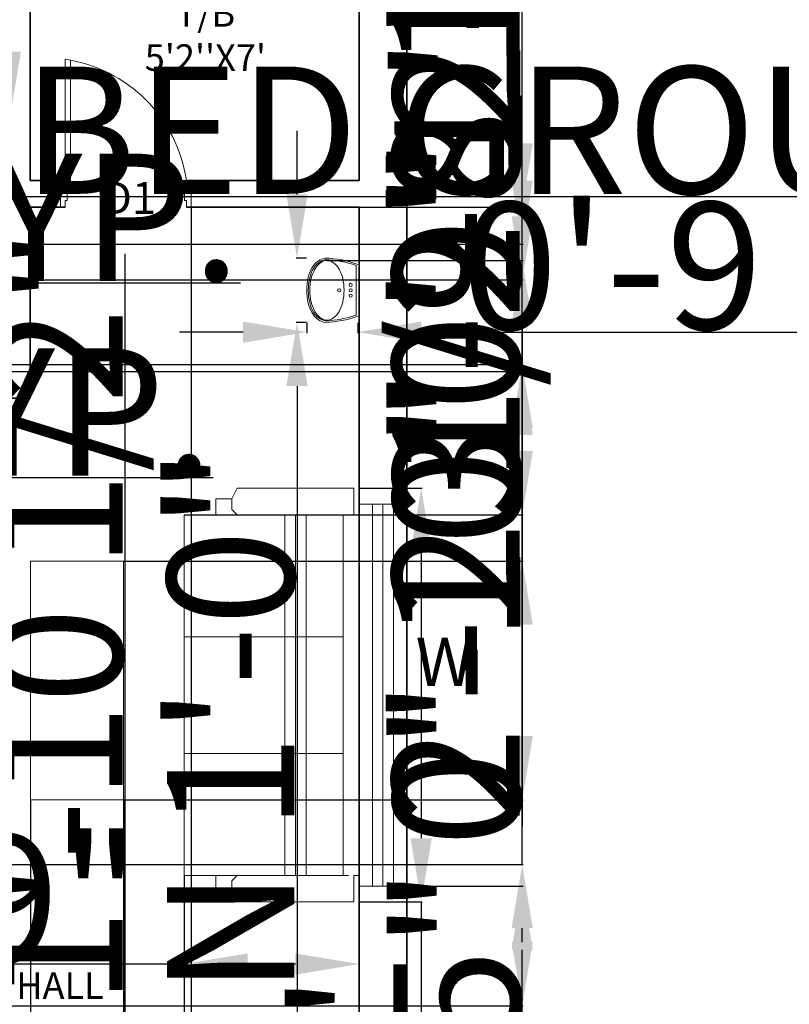
# Model space of a CAD drawing. Units: inches. Extents: x 2236 to 2927, y 1577 to 2452.
# Tile 6 of 9: x 2550 to 2695, y 1836 to 2021. Entities that reach past the tile are written whole.
import ezdxf

# ---------------------------------------------------------------- set-up
doc = ezdxf.new("R2010")
doc.units = ezdxf.units.IN
for name, color, linetype, lineweight in [('A-ANNO-DIMS', 2, 'Continuous', 18), ('A-ANNO-TEXT', 7, 'Continuous', 18), ('A-AREA-IDEN', 7, 'Continuous', 18), ('A-FLOR-FIXT', 9, 'Continuous', 18), ('A-FURN', 8, 'Continuous', 18), ('Doors', 150, 'Continuous', 18), ('Wall', 7, 'Continuous', 35), ('Windows', 162, 'Continuous', 18)]:
    doc.layers.add(name, color=color, linetype=linetype, lineweight=lineweight)
doc.styles.get("Standard").update_dxf_attribs({"font": 'arial.ttf'})
doc.dimstyles.get("Standard").update_dxf_attribs({"dimtxt": 24, "dimasz": 12, "dimexe": 0.18, "dimexo": 0.0625, "dimgap": 0.09, "dimtad": 1, "dimdec": 1, "dimzin": 0, "dimdsep": 46, "dimlunit": 4, "dimtxsty": 'Standard', "dimcen": 0.09, "dimadec": 0, "dimazin": 0, "dimtfac": 1, "dimtdec": 1, "dimtofl": 0, "dimtmove": 0, "dimatfit": 3, "dimfxl": 1, "dimtolj": 1, "dimtzin": 0, "dimarcsym": 0})

# ---------------------------------------------------------------- blocks, each defined once
blk = doc.blocks.new('wash-3')
at = {"color": 0, "linetype": 'ByBlock'}
blk.add_line((0.2303, -0.0146), (-0.2303, -0.0146), dxfattribs=at)
for centre in [(-0.05, -0.0656), (0, -0.0656), (0.05, -0.0656), (0, -0.1721)]:
    blk.add_circle(centre, 0.0148, dxfattribs=at)
for centre, radius, start, end in [((0.6901, -0.3398), 0.9908, 159.94105, 177.83899), ((0.6901, -0.3398), 0.9762, 160.53992, 177.73258), ((-0.6901, -0.3398), 0.9762, 2.26742, 19.46008), ((-0.6901, -0.3398), 0.9908, 2.16101, 20.05895), ((-0.0958, -0.3493), 0.2026, 119.83217, 144.15878), ((-0.038, -0.4501), 0.3188, 103.36192, 119.83217), ((0, -0.6101), 0.4833, 90, 103.36192), ((0, -0.6101), 0.4833, 76.63808, 90), ((0.038, -0.4501), 0.3188, 60.16783, 76.63808), ((0.0958, -0.3493), 0.2026, 35.84122, 60.16783), ((-0.1831, -0.2863), 0.095, 144.15878, 180), ((0.1831, -0.2863), 0.095, 0, 35.84122), ((-0.12, -0.2651), 0.1838, 191.74238, 233.41914), ((-0.12, -0.2651), 0.1692, 192.33583, 233.36097), ((-0.1831, -0.2863), 0.095, 180, 215.84122), ((-0.0958, -0.2233), 0.2026, 215.84122, 240.16783), ((0.0958, -0.2233), 0.2026, 299.83217, 324.15878), ((0.12, -0.2651), 0.1692, 306.63903, 347.66417), ((0.12, -0.2651), 0.1838, 306.58086, 348.25762), ((0.1831, -0.2863), 0.095, 324.15878, 0), ((-0.0958, -0.2233), 0.2319, 234.77185, 240.16783), ((-0.0958, -0.2233), 0.2173, 234.81756, 240.16783), ((-0.038, -0.1224), 0.3481, 240.16783, 256.63808), ((-0.038, -0.1224), 0.3335, 240.16783, 256.63808), ((-0.038, -0.1224), 0.3188, 240.16783, 256.63808), ((0, 0.0376), 0.4979, 256.63808, 270), ((0, 0.0376), 0.4833, 256.63808, 270), ((0, 0.0376), 0.4833, 270, 283.36192), ((0, 0.0376), 0.4979, 270, 283.36192), ((0.038, -0.1224), 0.3188, 283.36192, 299.83217), ((0.038, -0.1224), 0.3335, 283.36192, 299.83217), ((0.038, -0.1224), 0.3481, 283.36192, 299.83217), ((0.0958, -0.2233), 0.2173, 299.83217, 305.18244), ((0.0958, -0.2233), 0.2319, 299.83217, 305.22815), ((0, 0.0376), 0.5126, 256.63808, 270), ((0, 0.0376), 0.5126, 270, 283.36192)]:
    blk.add_arc(centre, radius, start, end, dxfattribs=at)
blk = doc.blocks.new('12PCOU13')
at = {"color": 0, "linetype": 'ByBlock'}
for p, q in [((24, 37), (24, 35)), ((23, 34), (2, 34)), ((3, -34), (3, 34)), ((10, 34), (10, -34)), ((12, 34), (12, -34)), ((14, 34), (14, -34)), ((24, 35), (23, 34)), ((27, 34), (23, 34)), ((33, 11), (3, 11)), ((33, -11), (3, -11)), ((23, -34), (2, -34)), ((27, -34), (23, -34)), ((24, -35), (23, -34)), ((24, -37), (24, -35))]:
    blk.add_line(p, q, dxfattribs=at)
blk.add_lwpolyline([(1, -39), (1, -34), (0, -34), (0, 34), (1, 34), (1, 39), (23, 39), (24, 37), (27, 37), (27, 34), (33, 34), (33, -34), (27, -34), (27, -37), (24, -37), (23, -39)], close=True, dxfattribs=at)
blk = doc.blocks.new('AP0B07')
for p, q in [((33.6, 96), (33.6, 978.8)), ((72, 96), (72, 972.3)), ((0, 96), (0, -96)), ((33.6, 96), (0, 96)), ((33.6, 48), (33.6, 96)), ((48, 48), (33.6, 48)), ((48, -48), (48, 48)), ((33.6, -96), (33.6, -48)), ((33.6, -48), (48, -48)), ((0, -96), (33.6, -96))]:
    blk.add_line(p, q)
blk.add_lwpolyline([(33.6, 96), (72, 96)])
blk.add_lwpolyline([(950, 96), (950, -96), (916.4, -96), (916.4, -48), (902, -48), (902, 48), (916.4, 48), (916.4, 96)], close=True)
blk.add_arc((-123.6, -61.2), 1051.8, 8.59637, 81.40363)
blk = doc.blocks.new('WIN-72IN')
for p, q in [((0, 6.5), (72, 6.5)), ((0, 4.5), (72, 4.5)), ((0, 2.5), (72, 2.5))]:
    blk.add_line(p, q)
blk.add_lwpolyline([(0, 9), (72, 9), (72, 0), (0, 0)], close=True)
blk = doc.blocks.new('*D17')
at = {"layer": 'A-ANNO-DIMS', "color": 0, "lineweight": -2, "transparency": 16777216}
for p, q in [((2405.85, 1971.79), (2393.85, 1971.79)), ((2417.85, 1972.28), (2417.85, 1971.61)), ((2420.99, 1972.28), (2420.99, 1971.61)), ((2432.99, 1971.79), (2591.46, 1971.79))]:
    blk.add_line(p, q, dxfattribs=at)
at = {"layer": 'A-ANNO-DIMS', "color": 0, "transparency": 16777216}
for points in [[(2405.85, 1973.79), (2405.85, 1969.79), (2417.85, 1971.79)], [(2432.99, 1973.79), (2432.99, 1969.79), (2420.99, 1971.79)]]:
    blk.add_solid(points, dxfattribs=at)
at = {"layer": 'Defpoints', "color": 0, "transparency": 16777216}
for p in [(2417.85, 1972.34), (2420.99, 1972.34), (2420.99, 1971.79)]:
    blk.add_point(p, dxfattribs=at)
at = {"layer": 'A-ANNO-DIMS', "color": 0, "transparency": 16777216, "insert": (2518.23, 1984.14), "char_height": 24, "attachment_point": 5}
blk.add_mtext('\\A1;0\'-3" TYP.', dxfattribs=at)
blk = doc.blocks.new('*D21')
at = {"layer": 'A-ANNO-DIMS', "color": 0, "lineweight": -2, "transparency": 16777216}
for p, q in [((2394.85, 1935.11), (2382.85, 1935.11)), ((2406.85, 1929.77), (2406.85, 1935.29)), ((2415.85, 1929.77), (2415.85, 1935.29)), ((2427.85, 1935.11), (2586.32, 1935.11))]:
    blk.add_line(p, q, dxfattribs=at)
at = {"layer": 'A-ANNO-DIMS', "color": 0, "transparency": 16777216}
for points in [[(2394.85, 1937.11), (2394.85, 1933.11), (2406.85, 1935.11)], [(2427.85, 1937.11), (2427.85, 1933.11), (2415.85, 1935.11)]]:
    blk.add_solid(points, dxfattribs=at)
at = {"layer": 'Defpoints', "color": 0, "transparency": 16777216}
for p in [(2415.85, 1935.11), (2406.85, 1929.71), (2415.85, 1929.71)]:
    blk.add_point(p, dxfattribs=at)
at = {"layer": 'A-ANNO-DIMS', "color": 0, "transparency": 16777216, "insert": (2513.08, 1947.45), "char_height": 24, "attachment_point": 5}
blk.add_mtext('\\A1;0\'-9" TYP.', dxfattribs=at)
blk = doc.blocks.new('*D22')
at = {"layer": 'A-ANNO-DIMS', "color": 0, "lineweight": -2, "transparency": 16777216}
for p, q in [((2514.42, 1977.96), (2514.42, 2358.7)), ((2518.53, 1977.96), (2514.24, 1977.96)), ((2514.42, 1962.08), (2514.42, 1965.96)), ((2518.53, 1950.08), (2514.24, 1950.08))]:
    blk.add_line(p, q, dxfattribs=at)
at = {"layer": 'A-ANNO-DIMS', "color": 0, "transparency": 16777216}
for points in [[(2512.42, 1965.96), (2516.42, 1965.96), (2514.42, 1977.96)], [(2512.42, 1962.08), (2516.42, 1962.08), (2514.42, 1950.08)]]:
    blk.add_solid(points, dxfattribs=at)
at = {"layer": 'Defpoints', "color": 0, "transparency": 16777216}
for p in [(2514.42, 1977.96), (2518.6, 1977.96), (2518.6, 1950.08)]:
    blk.add_point(p, dxfattribs=at)
at = {"layer": 'A-ANNO-DIMS', "color": 0, "transparency": 16777216, "insert": (2501.91, 2174.33), "char_height": 24, "attachment_point": 5, "rotation": 90}
blk.add_mtext('\\A1;ROOM DOOR 2\'-4" TYP.', dxfattribs=at)
blk = doc.blocks.new('*D26')
at = {"layer": 'A-ANNO-DIMS', "color": 0, "lineweight": -2, "transparency": 16777216}
for p, q in [((2602.14, 1988.47), (2602.14, 2000.47)), ((2603.9, 1976.47), (2601.96, 1976.47)), ((2603.9, 1964.32), (2601.96, 1964.32)), ((2602.14, 1952.32), (2602.14, 1767.47))]:
    blk.add_line(p, q, dxfattribs=at)
at = {"layer": 'A-ANNO-DIMS', "color": 0, "transparency": 16777216}
for points in [[(2600.14, 1988.47), (2604.14, 1988.47), (2602.14, 1976.47)], [(2600.14, 1952.32), (2604.14, 1952.32), (2602.14, 1964.32)]]:
    blk.add_solid(points, dxfattribs=at)
at = {"layer": 'Defpoints', "color": 0, "transparency": 16777216}
for p in [(2603.96, 1976.47), (2602.14, 1964.32), (2603.96, 1964.32)]:
    blk.add_point(p, dxfattribs=at)
at = {"layer": 'A-ANNO-DIMS', "color": 0, "transparency": 16777216, "insert": (2589.64, 1853.9), "char_height": 24, "attachment_point": 5, "rotation": 90}
blk.add_mtext('\\A1;BASIN 1\'-0"', dxfattribs=at)
blk = doc.blocks.new('*D27')
at = {"layer": 'A-ANNO-DIMS', "color": 0, "lineweight": -2, "transparency": 16777216}
for p, q in [((2603.96, 1964.26), (2603.96, 1962.32)), ((2613.58, 1964.26), (2613.58, 1962.32)), ((2591.96, 1962.5), (2579.96, 1962.5)), ((2625.58, 1962.5), (2757.48, 1962.5))]:
    blk.add_line(p, q, dxfattribs=at)
at = {"layer": 'A-ANNO-DIMS', "color": 0, "transparency": 16777216}
for points in [[(2591.96, 1964.5), (2591.96, 1960.5), (2603.96, 1962.5)], [(2625.58, 1964.5), (2625.58, 1960.5), (2613.58, 1962.5)]]:
    blk.add_solid(points, dxfattribs=at)
at = {"layer": 'Defpoints', "color": 0, "transparency": 16777216}
for p in [(2603.96, 1964.32), (2613.58, 1964.32), (2613.58, 1962.5)]:
    blk.add_point(p, dxfattribs=at)
at = {"layer": 'A-ANNO-DIMS', "color": 0, "transparency": 16777216, "insert": (2697.53, 1975), "char_height": 24, "attachment_point": 5}
blk.add_mtext('\\A1;0\'-9 1/2"', dxfattribs=at)
blk = doc.blocks.new('*D28')
at = {"layer": 'A-ANNO-DIMS', "color": 0, "lineweight": -2, "transparency": 16777216}
for p, q in [((2430.9, 2003.29), (2430.9, 1987.89)), ((2532.8, 2003.29), (2532.8, 1987.89)), ((2442.9, 1988.07), (2520.8, 1988.07)), ((2532.8, 1988.07), (2818.23, 1988.07))]:
    blk.add_line(p, q, dxfattribs=at)
at = {"layer": 'A-ANNO-DIMS', "color": 0, "transparency": 16777216}
for points in [[(2442.9, 1990.07), (2442.9, 1986.07), (2430.9, 1988.07)], [(2520.8, 1990.07), (2520.8, 1986.07), (2532.8, 1988.07)]]:
    blk.add_solid(points, dxfattribs=at)
at = {"layer": 'Defpoints', "color": 0, "transparency": 16777216}
for p in [(2430.9, 2003.35), (2532.8, 2003.35), (2532.8, 1988.07)]:
    blk.add_point(p, dxfattribs=at)
at = {"layer": 'A-ANNO-DIMS', "color": 0, "transparency": 16777216, "insert": (2681.51, 2000.57), "char_height": 24, "attachment_point": 5}
blk.add_mtext('\\A1;BED GROUP 8\'-6"', dxfattribs=at)
blk = doc.blocks.new('*D29')
at = {"layer": 'A-ANNO-DIMS', "color": 0, "lineweight": -2, "transparency": 16777216}
for p, q in [((2548.08, 2075.08), (2548.08, 2225.62)), ((2532.86, 2075.08), (2548.26, 2075.08)), ((2548.08, 2015.35), (2548.08, 2063.08)), ((2532.86, 2003.35), (2548.26, 2003.35))]:
    blk.add_line(p, q, dxfattribs=at)
at = {"layer": 'A-ANNO-DIMS', "color": 0, "transparency": 16777216}
for points in [[(2546.08, 2063.08), (2550.08, 2063.08), (2548.08, 2075.08)], [(2546.08, 2015.35), (2550.08, 2015.35), (2548.08, 2003.35)]]:
    blk.add_solid(points, dxfattribs=at)
at = {"layer": 'Defpoints', "color": 0, "transparency": 16777216}
for p in [(2532.8, 2075.08), (2548.08, 2075.08), (2532.8, 2003.35)]:
    blk.add_point(p, dxfattribs=at)
at = {"layer": 'A-ANNO-DIMS', "color": 0, "transparency": 16777216, "insert": (2535.58, 2156.35), "char_height": 24, "attachment_point": 5, "rotation": 90}
blk.add_mtext('\\A1;5\'-11 1/2"', dxfattribs=at)
blk = doc.blocks.new('*D32')
at = {"layer": 'A-ANNO-DIMS', "color": 0, "lineweight": -2, "transparency": 16777216}
for p, q in [((2613.91, 1933.08), (2625.73, 1933.08)), ((2625.55, 1921.08), (2625.55, 1867.08)), ((2613.91, 1855.08), (2625.73, 1855.08)), ((2625.55, 1855.08), (2625.55, 1678.61))]:
    blk.add_line(p, q, dxfattribs=at)
at = {"layer": 'A-ANNO-DIMS', "color": 0, "transparency": 16777216}
for points in [[(2623.55, 1921.08), (2627.55, 1921.08), (2625.55, 1933.08)], [(2623.55, 1867.08), (2627.55, 1867.08), (2625.55, 1855.08)]]:
    blk.add_solid(points, dxfattribs=at)
at = {"layer": 'Defpoints', "color": 0, "transparency": 16777216}
for p in [(2613.85, 1933.08), (2613.85, 1855.08), (2625.55, 1855.08)]:
    blk.add_point(p, dxfattribs=at)
at = {"layer": 'A-ANNO-DIMS', "color": 0, "transparency": 16777216, "insert": (2613.04, 1760.84), "char_height": 24, "attachment_point": 5, "rotation": 90}
blk.add_mtext('\\A1;SOFA 6\'-6"', dxfattribs=at)
blk = doc.blocks.new('*D33')
at = {"layer": 'A-ANNO-DIMS', "color": 0, "lineweight": -2, "transparency": 16777216}
for p, q in [((2580.85, 1855.01), (2580.85, 1843.2)), ((2613.85, 1855.01), (2613.85, 1843.2)), ((2580.85, 1843.38), (2504.46, 1843.38)), ((2601.85, 1843.38), (2592.85, 1843.38))]:
    blk.add_line(p, q, dxfattribs=at)
at = {"layer": 'A-ANNO-DIMS', "color": 0, "transparency": 16777216}
for points in [[(2592.85, 1845.38), (2592.85, 1841.38), (2580.85, 1843.38)], [(2601.85, 1845.38), (2601.85, 1841.38), (2613.85, 1843.38)]]:
    blk.add_solid(points, dxfattribs=at)
at = {"layer": 'Defpoints', "color": 0, "transparency": 16777216}
for p in [(2580.85, 1855.08), (2613.85, 1855.08), (2580.85, 1843.38)]:
    blk.add_point(p, dxfattribs=at)
at = {"layer": 'A-ANNO-DIMS', "color": 0, "transparency": 16777216, "insert": (2536.65, 1855.72), "char_height": 24, "attachment_point": 5}
blk.add_mtext('\\A1;2\'-9"', dxfattribs=at)
blk = doc.blocks.new('*D34')
at = {"layer": 'A-ANNO-DIMS', "color": 0, "lineweight": -2, "transparency": 16777216}
for p, q in [((2520.69, 1794.44), (2520.69, 1787.92)), ((2563.35, 1794.44), (2563.35, 1787.92)), ((2532.69, 1788.1), (2551.35, 1788.1)), ((2563.35, 1788.1), (2926.83, 1788.1))]:
    blk.add_line(p, q, dxfattribs=at)
at = {"layer": 'A-ANNO-DIMS', "color": 0, "transparency": 16777216}
for points in [[(2532.69, 1790.1), (2532.69, 1786.1), (2520.69, 1788.1)], [(2551.35, 1790.1), (2551.35, 1786.1), (2563.35, 1788.1)]]:
    blk.add_solid(points, dxfattribs=at)
at = {"layer": 'Defpoints', "color": 0, "transparency": 16777216}
for p in [(2520.69, 1794.5), (2563.35, 1794.5), (2563.35, 1788.1)]:
    blk.add_point(p, dxfattribs=at)
at = {"layer": 'A-ANNO-DIMS', "color": 0, "transparency": 16777216, "insert": (2751.09, 1800.62), "char_height": 24, "attachment_point": 5}
blk.add_mtext('\\A1;ENTRY DOOR 3\'-6 1/2"', dxfattribs=at)
blk = doc.blocks.new('*D35')
at = {"layer": 'A-ANNO-DIMS', "color": 0, "lineweight": -2, "transparency": 16777216}
for p, q in [((2569.75, 1828.98), (2569.75, 1977.27)), ((2563.41, 1816.98), (2569.93, 1816.98)), ((2563.41, 1794.5), (2569.93, 1794.5)), ((2569.75, 1782.5), (2569.75, 1770.5))]:
    blk.add_line(p, q, dxfattribs=at)
at = {"layer": 'A-ANNO-DIMS', "color": 0, "transparency": 16777216}
for points in [[(2567.75, 1828.98), (2571.75, 1828.98), (2569.75, 1816.98)], [(2567.75, 1782.5), (2571.75, 1782.5), (2569.75, 1794.5)]]:
    blk.add_solid(points, dxfattribs=at)
at = {"layer": 'Defpoints', "color": 0, "transparency": 16777216}
for p in [(2563.35, 1816.98), (2569.75, 1816.98), (2563.35, 1794.5)]:
    blk.add_point(p, dxfattribs=at)
at = {"layer": 'A-ANNO-DIMS', "color": 0, "transparency": 16777216, "insert": (2557.25, 1909.13), "char_height": 24, "attachment_point": 5, "rotation": 90}
blk.add_mtext('\\A1;1\'-10 1/2"', dxfattribs=at)
blk = doc.blocks.new('*D45')
at = {"layer": 'A-ANNO-DIMS', "color": 0, "lineweight": -2, "transparency": 16777216}
for p, q in [((2622.91, 1858.08), (2644.78, 1858.08)), ((2644.6, 1805.08), (2644.6, 1846.08)), ((2622.91, 1793.08), (2644.78, 1793.08))]:
    blk.add_line(p, q, dxfattribs=at)
at = {"layer": 'A-ANNO-DIMS', "color": 0, "transparency": 16777216}
for points in [[(2642.6, 1846.08), (2646.6, 1846.08), (2644.6, 1858.08)], [(2642.6, 1805.08), (2646.6, 1805.08), (2644.6, 1793.08)]]:
    blk.add_solid(points, dxfattribs=at)
at = {"layer": 'Defpoints', "color": 0, "transparency": 16777216}
for p in [(2622.85, 1858.08), (2644.6, 1858.08), (2622.85, 1793.08)]:
    blk.add_point(p, dxfattribs=at)
at = {"layer": 'A-ANNO-DIMS', "color": 0, "transparency": 16777216, "insert": (2632.3, 1825.58), "char_height": 24, "attachment_point": 5, "rotation": 90}
blk.add_mtext('\\A1;5\'-5"', dxfattribs=at)
blk = doc.blocks.new('*D48')
at = {"layer": 'A-ANNO-DIMS', "color": 0, "lineweight": -2, "transparency": 16777216}
for p, q in [((2524.86, 1915.51), (2524.86, 1702.15)), ((2533.86, 1915.51), (2533.86, 1702.15)), ((2512.86, 1702.33), (2500.86, 1702.33)), ((2545.86, 1702.33), (2621.84, 1702.33))]:
    blk.add_line(p, q, dxfattribs=at)
at = {"layer": 'A-ANNO-DIMS', "color": 0, "transparency": 16777216}
for points in [[(2512.86, 1704.33), (2512.86, 1700.33), (2524.86, 1702.33)], [(2545.86, 1704.33), (2545.86, 1700.33), (2533.86, 1702.33)]]:
    blk.add_solid(points, dxfattribs=at)
at = {"layer": 'Defpoints', "color": 0, "transparency": 16777216}
for p in [(2524.86, 1915.58), (2533.86, 1915.58), (2533.86, 1702.33)]:
    blk.add_point(p, dxfattribs=at)
at = {"layer": 'A-ANNO-DIMS', "color": 0, "transparency": 16777216, "insert": (2589.85, 1714.67), "char_height": 24, "attachment_point": 5}
blk.add_mtext('\\A1;0\'-9"', dxfattribs=at)
blk = doc.blocks.new('*D51')
at = {"layer": 'A-ANNO-DIMS', "color": 0, "lineweight": -2, "transparency": 16777216}
for p, q in [((2644.6, 1862.15), (2644.6, 1994.46)), ((2512.91, 1862.15), (2644.78, 1862.15)), ((2644.6, 1847.53), (2644.6, 1850.15)), ((2512.91, 1835.53), (2644.78, 1835.53))]:
    blk.add_line(p, q, dxfattribs=at)
at = {"layer": 'A-ANNO-DIMS', "color": 0, "transparency": 16777216}
for points in [[(2642.6, 1850.15), (2646.6, 1850.15), (2644.6, 1862.15)], [(2642.6, 1847.53), (2646.6, 1847.53), (2644.6, 1835.53)]]:
    blk.add_solid(points, dxfattribs=at)
at = {"layer": 'Defpoints', "color": 0, "transparency": 16777216}
for p in [(2512.85, 1862.15), (2644.6, 1862.15), (2512.85, 1835.53)]:
    blk.add_point(p, dxfattribs=at)
at = {"layer": 'A-ANNO-DIMS', "color": 0, "transparency": 16777216, "insert": (2632.1, 1934.31), "char_height": 24, "attachment_point": 5, "rotation": 90}
blk.add_mtext('\\A1;2\'-2 1/2"', dxfattribs=at)
blk = doc.blocks.new('*D53')
at = {"layer": 'A-ANNO-DIMS', "color": 0, "lineweight": -2, "transparency": 16777216}
for p, q in [((2644.6, 1991.08), (2644.6, 2067.46)), ((2515.94, 1979.08), (2644.78, 1979.08)), ((2515.94, 1955.08), (2644.78, 1955.08)), ((2644.6, 1943.08), (2644.6, 1931.08))]:
    blk.add_line(p, q, dxfattribs=at)
at = {"layer": 'A-ANNO-DIMS', "color": 0, "transparency": 16777216}
for points in [[(2642.6, 1991.08), (2646.6, 1991.08), (2644.6, 1979.08)], [(2642.6, 1943.08), (2646.6, 1943.08), (2644.6, 1955.08)]]:
    blk.add_solid(points, dxfattribs=at)
at = {"layer": 'Defpoints', "color": 0, "transparency": 16777216}
for p in [(2515.88, 1979.08), (2644.6, 1979.08), (2515.88, 1955.08)]:
    blk.add_point(p, dxfattribs=at)
at = {"layer": 'A-ANNO-DIMS', "color": 0, "transparency": 16777216, "insert": (2632.25, 2035.27), "char_height": 24, "attachment_point": 5, "rotation": 90}
blk.add_mtext('\\A1;2\'-0"', dxfattribs=at)
blk = doc.blocks.new('*D54')
at = {"layer": 'A-ANNO-DIMS', "color": 0, "lineweight": -2, "transparency": 16777216}
for p, q in [((2543.24, 1954.99), (2543.24, 1702.15)), ((2547.85, 1955.01), (2547.85, 1702.15)), ((2531.24, 1702.33), (2519.24, 1702.33)), ((2559.85, 1702.33), (2691.75, 1702.33))]:
    blk.add_line(p, q, dxfattribs=at)
at = {"layer": 'A-ANNO-DIMS', "color": 0, "transparency": 16777216}
for points in [[(2531.24, 1704.33), (2531.24, 1700.33), (2543.24, 1702.33)], [(2559.85, 1704.33), (2559.85, 1700.33), (2547.85, 1702.33)]]:
    blk.add_solid(points, dxfattribs=at)
at = {"layer": 'Defpoints', "color": 0, "transparency": 16777216}
for p in [(2543.24, 1955.06), (2547.85, 1955.08), (2547.85, 1702.33)]:
    blk.add_point(p, dxfattribs=at)
at = {"layer": 'A-ANNO-DIMS', "color": 0, "transparency": 16777216, "insert": (2631.8, 1714.83), "char_height": 24, "attachment_point": 5}
blk.add_mtext('\\A1;0\'-4 1/2"', dxfattribs=at)
blk = doc.blocks.new('*D55')
at = {"layer": 'A-ANNO-DIMS', "color": 0, "lineweight": -2, "transparency": 16777216}
for p, q in [((2582.18, 1986.01), (2582.18, 1702.15)), ((2613.85, 1986.01), (2613.85, 1702.15)), ((2594.18, 1702.33), (2601.85, 1702.33)), ((2613.85, 1702.33), (2746.16, 1702.33))]:
    blk.add_line(p, q, dxfattribs=at)
at = {"layer": 'A-ANNO-DIMS', "color": 0, "transparency": 16777216}
for points in [[(2594.18, 1704.33), (2594.18, 1700.33), (2582.18, 1702.33)], [(2601.85, 1704.33), (2601.85, 1700.33), (2613.85, 1702.33)]]:
    blk.add_solid(points, dxfattribs=at)
at = {"layer": 'Defpoints', "color": 0, "transparency": 16777216}
for p in [(2582.18, 1986.08), (2613.85, 1986.08), (2613.85, 1702.33)]:
    blk.add_point(p, dxfattribs=at)
at = {"layer": 'A-ANNO-DIMS', "color": 0, "transparency": 16777216, "insert": (2686, 1714.83), "char_height": 24, "attachment_point": 5}
blk.add_mtext('\\A1;2\'-7 1/2"', dxfattribs=at)
blk = doc.blocks.new('*D56')
at = {"layer": 'A-ANNO-DIMS', "color": 0, "lineweight": -2, "transparency": 16777216}
for p, q in [((2551.88, 1874.28), (2551.88, 1702.15)), ((2569.42, 1874.28), (2569.42, 1702.15)), ((2539.88, 1702.33), (2527.88, 1702.33)), ((2581.42, 1702.33), (2711.06, 1702.33))]:
    blk.add_line(p, q, dxfattribs=at)
at = {"layer": 'A-ANNO-DIMS', "color": 0, "transparency": 16777216}
for points in [[(2539.88, 1704.33), (2539.88, 1700.33), (2551.88, 1702.33)], [(2581.42, 1704.33), (2581.42, 1700.33), (2569.42, 1702.33)]]:
    blk.add_solid(points, dxfattribs=at)
at = {"layer": 'Defpoints', "color": 0, "transparency": 16777216}
for p in [(2551.88, 1874.34), (2569.42, 1874.34), (2569.42, 1702.33)]:
    blk.add_point(p, dxfattribs=at)
at = {"layer": 'A-ANNO-DIMS', "color": 0, "transparency": 16777216, "insert": (2652.24, 1714.83), "char_height": 24, "attachment_point": 5}
blk.add_mtext('\\A1;1\'-5 1/2"', dxfattribs=at)
blk = doc.blocks.new('*D57')
at = {"layer": 'A-ANNO-DIMS', "color": 0, "lineweight": -2, "transparency": 16777216}
for p, q in [((2644.6, 1919.34), (2644.6, 1995.3)), ((2569.48, 1919.34), (2644.78, 1919.34)), ((2644.6, 1886.34), (2644.6, 1907.34)), ((2569.48, 1874.34), (2644.78, 1874.34))]:
    blk.add_line(p, q, dxfattribs=at)
at = {"layer": 'A-ANNO-DIMS', "color": 0, "transparency": 16777216}
for points in [[(2642.6, 1907.34), (2646.6, 1907.34), (2644.6, 1919.34)], [(2642.6, 1886.34), (2646.6, 1886.34), (2644.6, 1874.34)]]:
    blk.add_solid(points, dxfattribs=at)
at = {"layer": 'Defpoints', "color": 0, "transparency": 16777216}
for p in [(2569.42, 1919.34), (2644.6, 1919.34), (2569.42, 1874.34)]:
    blk.add_point(p, dxfattribs=at)
at = {"layer": 'A-ANNO-DIMS', "color": 0, "transparency": 16777216, "insert": (2632.25, 1963.32), "char_height": 24, "attachment_point": 5, "rotation": 90}
blk.add_mtext('\\A1;3\'-9"', dxfattribs=at)
blk = doc.blocks.new('*D63')
at = {"layer": 'A-ANNO-DIMS', "color": 0, "lineweight": -2, "transparency": 16777216}
for p, q in [((2644.6, 1984.34), (2644.6, 2058.06)), ((2511.22, 1972.34), (2644.78, 1972.34)), ((2511.22, 1956.39), (2644.78, 1956.39)), ((2644.6, 1944.39), (2644.6, 1932.39))]:
    blk.add_line(p, q, dxfattribs=at)
at = {"layer": 'A-ANNO-DIMS', "color": 0, "transparency": 16777216}
for points in [[(2642.6, 1984.34), (2646.6, 1984.34), (2644.6, 1972.34)], [(2642.6, 1944.39), (2646.6, 1944.39), (2644.6, 1956.39)]]:
    blk.add_solid(points, dxfattribs=at)
at = {"layer": 'Defpoints', "color": 0, "transparency": 16777216}
for p in [(2511.16, 1972.34), (2644.6, 1972.34), (2511.16, 1956.39)]:
    blk.add_point(p, dxfattribs=at)
at = {"layer": 'A-ANNO-DIMS', "color": 0, "transparency": 16777216, "insert": (2632.46, 2027.2), "char_height": 24, "attachment_point": 5, "rotation": 90}
blk.add_mtext('\\A1;1\'-4"', dxfattribs=at)
blk = doc.blocks.new('*D64')
at = {"layer": 'A-ANNO-DIMS', "color": 0, "lineweight": -2, "transparency": 16777216}
for p, q in [((2569.42, 1874.28), (2569.42, 1702.15)), ((2580.85, 1860.01), (2580.85, 1702.15)), ((2557.42, 1702.33), (2545.42, 1702.33)), ((2592.85, 1702.33), (2743.4, 1702.33))]:
    blk.add_line(p, q, dxfattribs=at)
at = {"layer": 'A-ANNO-DIMS', "color": 0, "transparency": 16777216}
for points in [[(2557.42, 1704.33), (2557.42, 1700.33), (2569.42, 1702.33)], [(2592.85, 1704.33), (2592.85, 1700.33), (2580.85, 1702.33)]]:
    blk.add_solid(points, dxfattribs=at)
at = {"layer": 'Defpoints', "color": 0, "transparency": 16777216}
for p in [(2569.42, 1874.34), (2580.85, 1860.08), (2580.85, 1702.33)]:
    blk.add_point(p, dxfattribs=at)
at = {"layer": 'A-ANNO-DIMS', "color": 0, "transparency": 16777216, "insert": (2674.12, 1714.83), "char_height": 24, "attachment_point": 5}
blk.add_mtext('\\A1;0\'-11 1/2"', dxfattribs=at)
blk = doc.blocks.new('*D65')
at = {"layer": 'A-ANNO-DIMS', "color": 0, "lineweight": -2, "transparency": 16777216}
for p, q in [((2644.6, 1940.08), (2644.6, 2071.98)), ((2580.91, 1928.08), (2644.78, 1928.08)), ((2569.48, 1919.34), (2644.78, 1919.34)), ((2644.6, 1907.34), (2644.6, 1895.34))]:
    blk.add_line(p, q, dxfattribs=at)
at = {"layer": 'A-ANNO-DIMS', "color": 0, "transparency": 16777216}
for points in [[(2642.6, 1940.08), (2646.6, 1940.08), (2644.6, 1928.08)], [(2642.6, 1907.34), (2646.6, 1907.34), (2644.6, 1919.34)]]:
    blk.add_solid(points, dxfattribs=at)
at = {"layer": 'Defpoints', "color": 0, "transparency": 16777216}
for p in [(2580.85, 1928.08), (2644.6, 1928.08), (2569.42, 1919.34)]:
    blk.add_point(p, dxfattribs=at)
at = {"layer": 'A-ANNO-DIMS', "color": 0, "transparency": 16777216, "insert": (2632.1, 2012.03), "char_height": 24, "attachment_point": 5, "rotation": 90}
blk.add_mtext('\\A1;0\'-8 1/2"', dxfattribs=at)
blk = doc.blocks.new('*D67')
at = {"layer": 'A-ANNO-DIMS', "color": 0, "lineweight": -2, "transparency": 16777216}
for p, q in [((2644.6, 1998.08), (2644.6, 2010.08)), ((2613.91, 1986.08), (2644.78, 1986.08)), ((2607.85, 1976.03), (2644.78, 1976.03)), ((2644.6, 1964.03), (2644.6, 1869.4))]:
    blk.add_line(p, q, dxfattribs=at)
at = {"layer": 'A-ANNO-DIMS', "color": 0, "transparency": 16777216}
for points in [[(2642.6, 1998.08), (2646.6, 1998.08), (2644.6, 1986.08)], [(2642.6, 1964.03), (2646.6, 1964.03), (2644.6, 1976.03)]]:
    blk.add_solid(points, dxfattribs=at)
at = {"layer": 'Defpoints', "color": 0, "transparency": 16777216}
for p in [(2613.85, 1986.08), (2607.79, 1976.03), (2644.6, 1976.03)]:
    blk.add_point(p, dxfattribs=at)
at = {"layer": 'A-ANNO-DIMS', "color": 0, "transparency": 16777216, "insert": (2632.25, 1910.71), "char_height": 24, "attachment_point": 5, "rotation": 90}
blk.add_mtext('\\A1;0\'-10"', dxfattribs=at)

msp = doc.modelspace()

# ---------------------------------------------------------------- linework, layer by layer
at = {"layer": 'A-FURN'}
msp.add_lwpolyline([(2569.42, 1919.34), (2551.88, 1919.34), (2551.88, 1874.34), (2569.42, 1874.34)], close=True, dxfattribs=at)
at = {"layer": 'Wall'}
for p, q in [((2622.85, 2084.08), (2622.85, 1724.08)), ((2551.85, 2075.08), (2551.85, 1991.08)), ((2613.85, 2075.08), (2613.85, 1991.08)), ((2551.85, 1991.08), (2559.4, 1991.08)), ((2581.3, 1991.08), (2613.85, 1991.08)), ((2551.85, 1986.08), (2558.41, 1986.08)), ((2551.85, 1986.08), (2551.85, 1950.08)), ((2581.31, 1986.08), (2613.85, 1986.08)), ((2613.85, 1986.08), (2613.85, 1802.08)), ((2542.37, 1950.08), (2551.85, 1950.08))]:
    msp.add_line(p, q, dxfattribs=at)

# ---------------------------------------------------------------- block references
at = {"layer": 'A-FLOR-FIXT', "xscale": 20.25099649207013, "yscale": 20.25099649207013, "zscale": 20.25099649207013, "rotation": 270}
msp.add_blockref('wash-3', (2613.58, 1970.39), dxfattribs=at)
at = {"layer": 'A-FURN', "rotation": 180}
msp.add_blockref('12PCOU13', (2613.85, 1894.08), dxfattribs=at)
at = {"layer": 'Doors', "xscale": 0.0259404460783577, "yscale": 0.0259404460783577, "zscale": 0.0259404460783577}
msp.add_blockref('AP0B07', (2557.53, 1988.57), dxfattribs=at)
at = {"layer": 'Windows', "rotation": 90.00000000000188}
msp.add_blockref('WIN-72IN', (2622.85, 1858.08), dxfattribs=at)

# ---------------------------------------------------------------- texts
at = {"layer": 'A-ANNO-TEXT'}
for s, height, p in [('D1', 6, (2565.38, 1984.8)), ('W', 9.12, (2624.5, 1895.81))]:
    msp.add_text(s, height=height, dxfattribs=at).set_placement(p)
at = {"layer": 'A-AREA-IDEN', "char_height": 5, "attachment_point": 1}
for s, insert in [("\\pxqc;T/B\\P5'2''X7'", (2566.14, 2025.09)), ("\\pxqc;HALL\\P8'5''X15'5'", (2538.73, 1841.81))]:
    msp.add_mtext_dynamic_manual_height_columns(s, width=37.4353, gutter_width=12.5, heights=[0], dxfattribs=dict(at, insert=insert))

# ---------------------------------------------------------------- dimensions: what is measured, and where the dimension line sits
at = {"layer": 'A-ANNO-DIMS'}
for base, p1, p2, angle, text, picture, middle in [((2514.42, 1977.96), (2518.6, 1950.08), (2518.6, 1977.96), 90, 'ROOM DOOR <> TYP.', '*D22', (2501.91, 2174.33)), ((2602.1407, 1964.3191), (2603.9633, 1976.4697), (2603.9633, 1964.3191), 270, 'BASIN <>', '*D26', (2589.6414, 1853.8962)), ((2625.55, 1855.08), (2613.85, 1933.08), (2613.85, 1855.08), 270, 'SOFA <>', '*D32', (2613.04, 1760.84))]:
    dim = msp.add_linear_dim(base=base, p1=p1, p2=p2, angle=angle, text=text, dimstyle='Standard', override={"dimdec": 1, "dimlfac": 1, "dimrnd": 0, "dimzin": 1, "dimdsep": 46, "dimlunit": 4, "dimfrac": 2}, dxfattribs=at)
    dim.commit()
    dim.dimension.update_dxf_attribs({"geometry": picture, "text_midpoint": middle})
for base, p1, p2, angle, picture, middle in [((2548.08, 2075.08), (2532.8, 2003.35), (2532.8, 2075.08), 90, '*D29', (2535.58, 2156.35)), ((2644.6, 1928.08), (2569.42, 1919.34), (2580.85, 1928.08), 90, '*D65', (2632.1, 2012.03)), ((2644.6, 1979.08), (2515.88, 1955.08), (2515.88, 1979.08), 90, '*D53', (2632.25, 2035.27)), ((2644.598, 1972.3393), (2511.1585, 1956.3877), (2511.1585, 1972.3393), 90, '*D63', (2632.4589, 2027.1987)), ((2644.598, 1976.0252), (2613.848, 1986.0763), (2607.7851, 1976.0252), 90, '*D67', (2632.2543, 1910.7129)), ((2644.6, 1919.34), (2569.42, 1874.34), (2569.42, 1919.34), 90, '*D57', (2632.25, 1963.32)), ((2644.6, 1862.15), (2512.85, 1835.53), (2512.85, 1862.15), 90, '*D51', (2632.1, 1934.31)), ((2569.75, 1816.98), (2563.35, 1794.5), (2563.35, 1816.98), 90, '*D35', (2557.25, 1909.13)), ((2580.85, 1843.38), (2613.85, 1855.08), (2580.85, 1855.08), 180, '*D33', (2536.65, 1855.72)), ((2644.6, 1858.08), (2622.85, 1793.08), (2622.85, 1858.08), 90, '*D45', (2632.3, 1825.58))]:
    dim = msp.add_linear_dim(base=base, p1=p1, p2=p2, angle=angle, dimstyle='Standard', override={"dimdec": 1, "dimlfac": 1, "dimrnd": 0, "dimzin": 1, "dimdsep": 46, "dimlunit": 4, "dimfrac": 2}, dxfattribs=at)
    dim.commit()
    dim.dimension.update_dxf_attribs({"geometry": picture, "text_midpoint": middle})
for base, p1, p2, text, picture, middle in [((2532.8, 1988.07), (2430.9, 2003.35), (2532.8, 2003.35), 'BED GROUP <>', '*D28', (2681.51, 2000.57)), ((2420.99, 1971.79), (2417.85, 1972.34), (2420.99, 1972.34), '<> TYP.', '*D17', (2518.23, 1984.14)), ((2415.85, 1935.11), (2406.85, 1929.71), (2415.85, 1929.71), '<> TYP.', '*D21', (2513.08, 1947.45)), ((2563.35, 1788.1), (2520.69, 1794.5), (2563.35, 1794.5), 'ENTRY DOOR <>', '*D34', (2751.09, 1800.62))]:
    dim = msp.add_linear_dim(base=base, p1=p1, p2=p2, text=text, dimstyle='Standard', override={"dimdec": 1, "dimlfac": 1, "dimrnd": 0, "dimzin": 1, "dimdsep": 46, "dimlunit": 4, "dimfrac": 2}, dxfattribs=at)
    dim.commit()
    dim.dimension.update_dxf_attribs({"geometry": picture, "text_midpoint": middle})
for base, p1, p2, picture, middle in [((2613.58, 1962.5), (2603.96, 1964.32), (2613.58, 1964.32), '*D27', (2697.53, 1975)), ((2613.85, 1702.33), (2582.18, 1986.08), (2613.85, 1986.08), '*D55', (2686, 1714.83)), ((2547.85, 1702.33), (2543.24, 1955.06), (2547.85, 1955.08), '*D54', (2631.8, 1714.83)), ((2533.86, 1702.33), (2524.86, 1915.58), (2533.86, 1915.58), '*D48', (2589.85, 1714.67)), ((2569.42, 1702.33), (2551.88, 1874.34), (2569.42, 1874.34), '*D56', (2652.24, 1714.83)), ((2580.85, 1702.33), (2569.42, 1874.34), (2580.85, 1860.08), '*D64', (2674.12, 1714.83))]:
    dim = msp.add_linear_dim(base=base, p1=p1, p2=p2, dimstyle='Standard', override={"dimdec": 1, "dimlfac": 1, "dimrnd": 0, "dimzin": 1, "dimdsep": 46, "dimlunit": 4, "dimfrac": 2}, dxfattribs=at)
    dim.commit()
    dim.dimension.update_dxf_attribs({"geometry": picture, "text_midpoint": middle})

doc.saveas('drawing.dxf')
